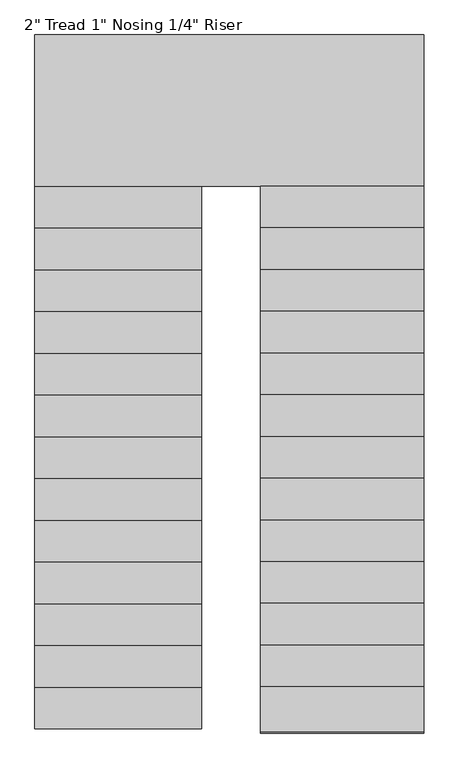
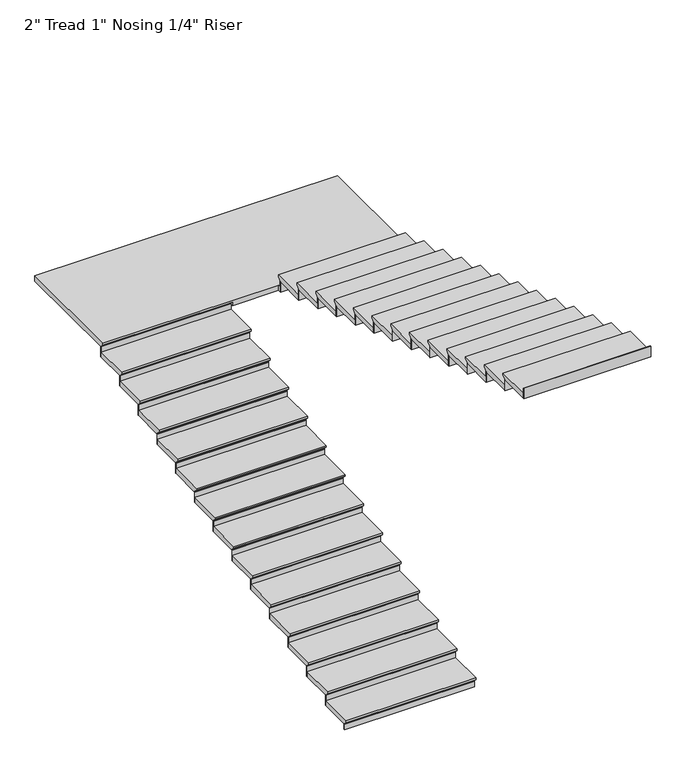
"""IFC4 building model written with IfcOpenShell, lengths in millimetres: stair flight geometry."""

from ifc_helpers import new_model, si_unit, origin, place, context, project, spatial, faceted_brep, source, transform, mapped, element, save


def stair_flight_f733c31e(model_context):
    return source(origin(), model_context, "Body", "Brep", [
        faceted_brep([(-629.5987998, 2564.5067329, 9685.5642857), (-629.5987998, 2564.5067329, 9704.6142857), (-1848.7987998, 2564.5067329, 9704.6142857), (-1848.7987998, 2564.5067329, 9685.5642857), (-629.5987998, 2589.9067329, 9660.1642857), (-1848.7987998, 2589.9067329, 9660.1642857), (-629.5987998, 2894.7067329, 9704.6142857), (-1848.7987998, 2894.7067329, 9704.6142857), (-1848.7987998, 2589.9067329, 9653.8142857), (-1848.7987998, 2894.7067329, 9653.8142857), (-629.5987998, 2894.7067329, 9653.8142857), (-629.5987998, 2589.9067329, 9653.8142857)], [[[0, 1, 2, 3]], [[4, 0, 3, 5]], [[2, 1, 6, 7]], [[8, 9, 10, 11]], [[2, 7, 9, 8, 5, 3]], [[8, 11, 4, 5]], [[6, 1, 0, 4, 11, 10]], [[7, 6, 10, 9]]]),
        faceted_brep([(-629.5987998, 2589.9067329, 9653.8142857), (-629.5987998, 2589.9067329, 9601.2), (-629.5987998, 2596.2567329, 9601.2), (-629.5987998, 2596.2567329, 9653.8142857), (-1848.7987998, 2589.9067329, 9653.8142857), (-1848.7987998, 2596.2567329, 9653.8142857), (-1848.7987998, 2596.2567329, 9601.2), (-1848.7987998, 2589.9067329, 9601.2)], [[[0, 1, 2, 3]], [[4, 5, 6, 7]], [[1, 0, 4, 7]], [[2, 1, 7, 6]], [[3, 2, 6, 5]], [[0, 3, 5, 4]]]),
        faceted_brep([(-629.5987998, 2894.7067329, 9757.2285714), (-629.5987998, 2894.7067329, 9653.8142857), (-629.5987998, 2901.0567329, 9653.8142857), (-629.5987998, 2901.0567329, 9757.2285714), (-1848.7987998, 2894.7067329, 9757.2285714), (-1848.7987998, 2901.0567329, 9757.2285714), (-1848.7987998, 2901.0567329, 9653.8142857), (-1848.7987998, 2894.7067329, 9653.8142857)], [[[0, 1, 2, 3]], [[4, 5, 6, 7]], [[1, 0, 4, 7]], [[2, 1, 7, 6]], [[3, 2, 6, 5]], [[0, 3, 5, 4]]]),
        faceted_brep([(-1848.7987998, 2869.3067329, 9808.0285714), (-629.5987998, 2869.3067329, 9808.0285714), (-629.5987998, 3199.5067329, 9808.0285714), (-1848.7987998, 3199.5067329, 9808.0285714), (-1848.7987998, 2894.7067329, 9757.2285714), (-1848.7987998, 3199.5067329, 9757.2285714), (-629.5987998, 3199.5067329, 9757.2285714), (-629.5987998, 2894.7067329, 9757.2285714), (-1848.7987998, 2894.7067329, 9763.5785714), (-1848.7987998, 2869.3067329, 9788.9785714), (-629.5987998, 2894.7067329, 9763.5785714), (-629.5987998, 2869.3067329, 9788.9785714)], [[[0, 1, 2, 3]], [[4, 5, 6, 7]], [[0, 3, 5, 4, 8, 9]], [[4, 7, 10, 8]], [[2, 1, 11, 10, 7, 6]], [[3, 2, 6, 5]], [[11, 1, 0, 9]], [[10, 11, 9, 8]]]),
        faceted_brep([(-629.5987998, 3199.5067329, 9860.6428571), (-629.5987998, 3199.5067329, 9757.2285714), (-629.5987998, 3205.8567329, 9757.2285714), (-629.5987998, 3205.8567329, 9860.6428571), (-1848.7987998, 3199.5067329, 9860.6428571), (-1848.7987998, 3205.8567329, 9860.6428571), (-1848.7987998, 3205.8567329, 9757.2285714), (-1848.7987998, 3199.5067329, 9757.2285714)], [[[0, 1, 2, 3]], [[4, 5, 6, 7]], [[1, 0, 4, 7]], [[2, 1, 7, 6]], [[3, 2, 6, 5]], [[0, 3, 5, 4]]]),
        faceted_brep([(-1848.7987998, 3174.1067329, 9911.4428571), (-629.5987998, 3174.1067329, 9911.4428571), (-629.5987998, 3504.3067329, 9911.4428571), (-1848.7987998, 3504.3067329, 9911.4428571), (-1848.7987998, 3199.5067329, 9860.6428571), (-1848.7987998, 3504.3067329, 9860.6428571), (-629.5987998, 3504.3067329, 9860.6428571), (-629.5987998, 3199.5067329, 9860.6428571), (-1848.7987998, 3199.5067329, 9866.9928571), (-1848.7987998, 3174.1067329, 9892.3928571), (-629.5987998, 3199.5067329, 9866.9928571), (-629.5987998, 3174.1067329, 9892.3928571)], [[[0, 1, 2, 3]], [[4, 5, 6, 7]], [[0, 3, 5, 4, 8, 9]], [[4, 7, 10, 8]], [[2, 1, 11, 10, 7, 6]], [[3, 2, 6, 5]], [[11, 1, 0, 9]], [[10, 11, 9, 8]]]),
        faceted_brep([(-629.5987998, 3504.3067329, 9964.0571429), (-629.5987998, 3504.3067329, 9860.6428571), (-629.5987998, 3510.6567329, 9860.6428571), (-629.5987998, 3510.6567329, 9964.0571429), (-1848.7987998, 3504.3067329, 9964.0571429), (-1848.7987998, 3510.6567329, 9964.0571429), (-1848.7987998, 3510.6567329, 9860.6428571), (-1848.7987998, 3504.3067329, 9860.6428571)], [[[0, 1, 2, 3]], [[4, 5, 6, 7]], [[1, 0, 4, 7]], [[2, 1, 7, 6]], [[3, 2, 6, 5]], [[0, 3, 5, 4]]]),
        faceted_brep([(-1848.7987998, 3478.9067329, 10014.8571429), (-629.5987998, 3478.9067329, 10014.8571429), (-629.5987998, 3809.1067329, 10014.8571429), (-1848.7987998, 3809.1067329, 10014.8571429), (-1848.7987998, 3504.3067329, 9964.0571429), (-1848.7987998, 3809.1067329, 9964.0571429), (-629.5987998, 3809.1067329, 9964.0571429), (-629.5987998, 3504.3067329, 9964.0571429), (-1848.7987998, 3504.3067329, 9970.4071429), (-1848.7987998, 3478.9067329, 9995.8071429), (-629.5987998, 3504.3067329, 9970.4071429), (-629.5987998, 3478.9067329, 9995.8071429)], [[[0, 1, 2, 3]], [[4, 5, 6, 7]], [[0, 3, 5, 4, 8, 9]], [[4, 7, 10, 8]], [[2, 1, 11, 10, 7, 6]], [[3, 2, 6, 5]], [[11, 1, 0, 9]], [[10, 11, 9, 8]]]),
        faceted_brep([(-629.5987998, 3809.1067329, 10067.4714286), (-629.5987998, 3809.1067329, 9964.0571429), (-629.5987998, 3815.4567329, 9964.0571429), (-629.5987998, 3815.4567329, 10067.4714286), (-1848.7987998, 3809.1067329, 10067.4714286), (-1848.7987998, 3815.4567329, 10067.4714286), (-1848.7987998, 3815.4567329, 9964.0571429), (-1848.7987998, 3809.1067329, 9964.0571429)], [[[0, 1, 2, 3]], [[4, 5, 6, 7]], [[1, 0, 4, 7]], [[2, 1, 7, 6]], [[3, 2, 6, 5]], [[0, 3, 5, 4]]]),
        faceted_brep([(-1848.7987998, 3783.7067329, 10118.2714286), (-629.5987998, 3783.7067329, 10118.2714286), (-629.5987998, 4113.9067329, 10118.2714286), (-1848.7987998, 4113.9067329, 10118.2714286), (-1848.7987998, 3809.1067329, 10067.4714286), (-1848.7987998, 4113.9067329, 10067.4714286), (-629.5987998, 4113.9067329, 10067.4714286), (-629.5987998, 3809.1067329, 10067.4714286), (-1848.7987998, 3809.1067329, 10073.8214286), (-1848.7987998, 3783.7067329, 10099.2214286), (-629.5987998, 3809.1067329, 10073.8214286), (-629.5987998, 3783.7067329, 10099.2214286)], [[[0, 1, 2, 3]], [[4, 5, 6, 7]], [[0, 3, 5, 4, 8, 9]], [[4, 7, 10, 8]], [[2, 1, 11, 10, 7, 6]], [[3, 2, 6, 5]], [[11, 1, 0, 9]], [[10, 11, 9, 8]]]),
        faceted_brep([(-629.5987998, 4113.9067329, 10170.8857143), (-629.5987998, 4113.9067329, 10067.4714286), (-629.5987998, 4120.2567329, 10067.4714286), (-629.5987998, 4120.2567329, 10170.8857143), (-1848.7987998, 4113.9067329, 10170.8857143), (-1848.7987998, 4120.2567329, 10170.8857143), (-1848.7987998, 4120.2567329, 10067.4714286), (-1848.7987998, 4113.9067329, 10067.4714286)], [[[0, 1, 2, 3]], [[4, 5, 6, 7]], [[1, 0, 4, 7]], [[2, 1, 7, 6]], [[3, 2, 6, 5]], [[0, 3, 5, 4]]]),
        faceted_brep([(-1848.7987998, 4088.5067329, 10221.6857143), (-629.5987998, 4088.5067329, 10221.6857143), (-629.5987998, 4418.7067329, 10221.6857143), (-1848.7987998, 4418.7067329, 10221.6857143), (-1848.7987998, 4113.9067329, 10170.8857143), (-1848.7987998, 4418.7067329, 10170.8857143), (-629.5987998, 4418.7067329, 10170.8857143), (-629.5987998, 4113.9067329, 10170.8857143), (-1848.7987998, 4113.9067329, 10177.2357143), (-1848.7987998, 4088.5067329, 10202.6357143), (-629.5987998, 4113.9067329, 10177.2357143), (-629.5987998, 4088.5067329, 10202.6357143)], [[[0, 1, 2, 3]], [[4, 5, 6, 7]], [[0, 3, 5, 4, 8, 9]], [[4, 7, 10, 8]], [[2, 1, 11, 10, 7, 6]], [[3, 2, 6, 5]], [[11, 1, 0, 9]], [[10, 11, 9, 8]]]),
        faceted_brep([(-629.5987998, 4418.7067329, 10274.3), (-629.5987998, 4418.7067329, 10170.8857143), (-629.5987998, 4425.0567329, 10170.8857143), (-629.5987998, 4425.0567329, 10274.3), (-1848.7987998, 4418.7067329, 10274.3), (-1848.7987998, 4425.0567329, 10274.3), (-1848.7987998, 4425.0567329, 10170.8857143), (-1848.7987998, 4418.7067329, 10170.8857143)], [[[0, 1, 2, 3]], [[4, 5, 6, 7]], [[1, 0, 4, 7]], [[2, 1, 7, 6]], [[3, 2, 6, 5]], [[0, 3, 5, 4]]]),
        faceted_brep([(-1848.7987998, 4393.3067329, 10325.1), (-629.5987998, 4393.3067329, 10325.1), (-629.5987998, 4723.5067329, 10325.1), (-1848.7987998, 4723.5067329, 10325.1), (-1848.7987998, 4418.7067329, 10274.3), (-1848.7987998, 4723.5067329, 10274.3), (-629.5987998, 4723.5067329, 10274.3), (-629.5987998, 4418.7067329, 10274.3), (-1848.7987998, 4418.7067329, 10280.65), (-1848.7987998, 4393.3067329, 10306.05), (-629.5987998, 4418.7067329, 10280.65), (-629.5987998, 4393.3067329, 10306.05)], [[[0, 1, 2, 3]], [[4, 5, 6, 7]], [[0, 3, 5, 4, 8, 9]], [[4, 7, 10, 8]], [[2, 1, 11, 10, 7, 6]], [[3, 2, 6, 5]], [[11, 1, 0, 9]], [[10, 11, 9, 8]]]),
        faceted_brep([(-629.5987998, 4723.5067329, 10377.7142857), (-629.5987998, 4723.5067329, 10274.3), (-629.5987998, 4729.8567329, 10274.3), (-629.5987998, 4729.8567329, 10377.7142857), (-1848.7987998, 4723.5067329, 10377.7142857), (-1848.7987998, 4729.8567329, 10377.7142857), (-1848.7987998, 4729.8567329, 10274.3), (-1848.7987998, 4723.5067329, 10274.3)], [[[0, 1, 2, 3]], [[4, 5, 6, 7]], [[1, 0, 4, 7]], [[2, 1, 7, 6]], [[3, 2, 6, 5]], [[0, 3, 5, 4]]]),
        faceted_brep([(-1848.7987998, 4698.1067329, 10428.5142857), (-629.5987998, 4698.1067329, 10428.5142857), (-629.5987998, 5028.3067329, 10428.5142857), (-1848.7987998, 5028.3067329, 10428.5142857), (-1848.7987998, 4723.5067329, 10377.7142857), (-1848.7987998, 5028.3067329, 10377.7142857), (-629.5987998, 5028.3067329, 10377.7142857), (-629.5987998, 4723.5067329, 10377.7142857), (-1848.7987998, 4723.5067329, 10384.0642857), (-1848.7987998, 4698.1067329, 10409.4642857), (-629.5987998, 4723.5067329, 10384.0642857), (-629.5987998, 4698.1067329, 10409.4642857)], [[[0, 1, 2, 3]], [[4, 5, 6, 7]], [[0, 3, 5, 4, 8, 9]], [[4, 7, 10, 8]], [[2, 1, 11, 10, 7, 6]], [[3, 2, 6, 5]], [[11, 1, 0, 9]], [[10, 11, 9, 8]]]),
        faceted_brep([(-629.5987998, 5028.3067329, 10481.1285714), (-629.5987998, 5028.3067329, 10377.7142857), (-629.5987998, 5034.6567329, 10377.7142857), (-629.5987998, 5034.6567329, 10481.1285714), (-1848.7987998, 5028.3067329, 10481.1285714), (-1848.7987998, 5034.6567329, 10481.1285714), (-1848.7987998, 5034.6567329, 10377.7142857), (-1848.7987998, 5028.3067329, 10377.7142857)], [[[0, 1, 2, 3]], [[4, 5, 6, 7]], [[1, 0, 4, 7]], [[2, 1, 7, 6]], [[3, 2, 6, 5]], [[0, 3, 5, 4]]]),
        faceted_brep([(-1848.7987998, 5002.9067329, 10531.9285714), (-629.5987998, 5002.9067329, 10531.9285714), (-629.5987998, 5333.1067329, 10531.9285714), (-1848.7987998, 5333.1067329, 10531.9285714), (-1848.7987998, 5028.3067329, 10481.1285714), (-1848.7987998, 5333.1067329, 10481.1285714), (-629.5987998, 5333.1067329, 10481.1285714), (-629.5987998, 5028.3067329, 10481.1285714), (-1848.7987998, 5028.3067329, 10487.4785714), (-1848.7987998, 5002.9067329, 10512.8785714), (-629.5987998, 5028.3067329, 10487.4785714), (-629.5987998, 5002.9067329, 10512.8785714)], [[[0, 1, 2, 3]], [[4, 5, 6, 7]], [[0, 3, 5, 4, 8, 9]], [[4, 7, 10, 8]], [[2, 1, 11, 10, 7, 6]], [[3, 2, 6, 5]], [[11, 1, 0, 9]], [[10, 11, 9, 8]]]),
        faceted_brep([(-629.5987998, 5333.1067329, 10584.5428571), (-629.5987998, 5333.1067329, 10481.1285714), (-629.5987998, 5339.4567329, 10481.1285714), (-629.5987998, 5339.4567329, 10584.5428571), (-1848.7987998, 5333.1067329, 10584.5428571), (-1848.7987998, 5339.4567329, 10584.5428571), (-1848.7987998, 5339.4567329, 10481.1285714), (-1848.7987998, 5333.1067329, 10481.1285714)], [[[0, 1, 2, 3]], [[4, 5, 6, 7]], [[1, 0, 4, 7]], [[2, 1, 7, 6]], [[3, 2, 6, 5]], [[0, 3, 5, 4]]]),
        faceted_brep([(-1848.7987998, 5307.7067329, 10635.3428571), (-629.5987998, 5307.7067329, 10635.3428571), (-629.5987998, 5637.9067329, 10635.3428571), (-1848.7987998, 5637.9067329, 10635.3428571), (-1848.7987998, 5333.1067329, 10584.5428571), (-1848.7987998, 5637.9067329, 10584.5428571), (-629.5987998, 5637.9067329, 10584.5428571), (-629.5987998, 5333.1067329, 10584.5428571), (-1848.7987998, 5333.1067329, 10590.8928571), (-1848.7987998, 5307.7067329, 10616.2928571), (-629.5987998, 5333.1067329, 10590.8928571), (-629.5987998, 5307.7067329, 10616.2928571)], [[[0, 1, 2, 3]], [[4, 5, 6, 7]], [[0, 3, 5, 4, 8, 9]], [[4, 7, 10, 8]], [[2, 1, 11, 10, 7, 6]], [[3, 2, 6, 5]], [[11, 1, 0, 9]], [[10, 11, 9, 8]]]),
        faceted_brep([(-629.5987998, 5637.9067329, 10687.9571429), (-629.5987998, 5637.9067329, 10584.5428571), (-629.5987998, 5644.2567329, 10584.5428571), (-629.5987998, 5644.2567329, 10687.9571429), (-1848.7987998, 5637.9067329, 10687.9571429), (-1848.7987998, 5644.2567329, 10687.9571429), (-1848.7987998, 5644.2567329, 10584.5428571), (-1848.7987998, 5637.9067329, 10584.5428571)], [[[0, 1, 2, 3]], [[4, 5, 6, 7]], [[1, 0, 4, 7]], [[2, 1, 7, 6]], [[3, 2, 6, 5]], [[0, 3, 5, 4]]]),
        faceted_brep([(-1848.7987998, 5612.5067329, 10738.7571429), (-629.5987998, 5612.5067329, 10738.7571429), (-629.5987998, 5942.7067329, 10738.7571429), (-1848.7987998, 5942.7067329, 10738.7571429), (-1848.7987998, 5637.9067329, 10687.9571429), (-1848.7987998, 5942.7067329, 10687.9571429), (-629.5987998, 5942.7067329, 10687.9571429), (-629.5987998, 5637.9067329, 10687.9571429), (-1848.7987998, 5637.9067329, 10694.3071429), (-1848.7987998, 5612.5067329, 10719.7071429), (-629.5987998, 5637.9067329, 10694.3071429), (-629.5987998, 5612.5067329, 10719.7071429)], [[[0, 1, 2, 3]], [[4, 5, 6, 7]], [[0, 3, 5, 4, 8, 9]], [[4, 7, 10, 8]], [[2, 1, 11, 10, 7, 6]], [[3, 2, 6, 5]], [[11, 1, 0, 9]], [[10, 11, 9, 8]]]),
        faceted_brep([(-629.5987998, 5942.7067329, 10791.3714286), (-629.5987998, 5942.7067329, 10687.9571429), (-629.5987998, 5949.0567329, 10687.9571429), (-629.5987998, 5949.0567329, 10791.3714286), (-1848.7987998, 5942.7067329, 10791.3714286), (-1848.7987998, 5949.0567329, 10791.3714286), (-1848.7987998, 5949.0567329, 10687.9571429), (-1848.7987998, 5942.7067329, 10687.9571429)], [[[0, 1, 2, 3]], [[4, 5, 6, 7]], [[1, 0, 4, 7]], [[2, 1, 7, 6]], [[3, 2, 6, 5]], [[0, 3, 5, 4]]]),
        faceted_brep([(-1848.7987998, 5917.3067329, 10842.1714286), (-629.5987998, 5917.3067329, 10842.1714286), (-629.5987998, 6247.5067329, 10842.1714286), (-1848.7987998, 6247.5067329, 10842.1714286), (-1848.7987998, 5942.7067329, 10791.3714286), (-1848.7987998, 6247.5067329, 10791.3714286), (-629.5987998, 6247.5067329, 10791.3714286), (-629.5987998, 5942.7067329, 10791.3714286), (-1848.7987998, 5942.7067329, 10797.7214286), (-1848.7987998, 5917.3067329, 10823.1214286), (-629.5987998, 5942.7067329, 10797.7214286), (-629.5987998, 5917.3067329, 10823.1214286)], [[[0, 1, 2, 3]], [[4, 5, 6, 7]], [[0, 3, 5, 4, 8, 9]], [[4, 7, 10, 8]], [[2, 1, 11, 10, 7, 6]], [[3, 2, 6, 5]], [[11, 1, 0, 9]], [[10, 11, 9, 8]]]),
        faceted_brep([(-629.5987998, 6247.5067329, 10894.7857143), (-629.5987998, 6247.5067329, 10791.3714286), (-629.5987998, 6253.8567329, 10791.3714286), (-629.5987998, 6253.8567329, 10894.7857143), (-1848.7987998, 6247.5067329, 10894.7857143), (-1848.7987998, 6253.8567329, 10894.7857143), (-1848.7987998, 6253.8567329, 10791.3714286), (-1848.7987998, 6247.5067329, 10791.3714286)], [[[0, 1, 2, 3]], [[4, 5, 6, 7]], [[1, 0, 4, 7]], [[2, 1, 7, 6]], [[3, 2, 6, 5]], [[0, 3, 5, 4]]]),
        faceted_brep([(-1848.7987998, 6222.1067329, 10945.5857143), (-629.5987998, 6222.1067329, 10945.5857143), (-629.5987998, 6552.3067329, 10945.5857143), (-1848.7987998, 6552.3067329, 10945.5857143), (-1848.7987998, 6247.5067329, 10894.7857143), (-1848.7987998, 6552.3067329, 10894.7857143), (-629.5987998, 6552.3067329, 10894.7857143), (-629.5987998, 6247.5067329, 10894.7857143), (-1848.7987998, 6247.5067329, 10901.1357143), (-1848.7987998, 6222.1067329, 10926.5357143), (-629.5987998, 6247.5067329, 10901.1357143), (-629.5987998, 6222.1067329, 10926.5357143)], [[[0, 1, 2, 3]], [[4, 5, 6, 7]], [[0, 3, 5, 4, 8, 9]], [[4, 7, 10, 8]], [[2, 1, 11, 10, 7, 6]], [[3, 2, 6, 5]], [[11, 1, 0, 9]], [[10, 11, 9, 8]]]),
        faceted_brep([(-629.5987998, 6552.3067329, 10998.2), (-629.5987998, 6552.3067329, 10894.7857143), (-629.5987998, 6558.6567329, 10894.7857143), (-629.5987998, 6558.6567329, 10998.2), (-1848.7987998, 6552.3067329, 10998.2), (-1848.7987998, 6558.6567329, 10998.2), (-1848.7987998, 6558.6567329, 10894.7857143), (-1848.7987998, 6552.3067329, 10894.7857143)], [[[0, 1, 2, 3]], [[4, 5, 6, 7]], [[1, 0, 4, 7]], [[2, 1, 7, 6]], [[3, 2, 6, 5]], [[0, 3, 5, 4]]]),
        faceted_brep([(996.0012002, 6501.5067329, 11049.0), (996.0012002, 7631.8067329, 11049.0), (-1848.7987998, 7631.8067329, 11049.0), (-1848.7987998, 6526.9067329, 11049.0), (-197.7987915, 6526.9067329, 11049.0), (-197.7987915, 6501.5067329, 11049.0), (996.0012002, 7631.8067329, 10998.2), (996.0012002, 6501.5067329, 10998.2), (-197.7987915, 6501.5067329, 10998.2), (-197.7987915, 6526.9067329, 10998.2), (-629.5987998, 6526.9067329, 10998.2), (-629.5987998, 6552.3067329, 10998.2), (-1848.7987998, 6552.3067329, 10998.2), (-1848.7987998, 7631.8067329, 10998.2), (-629.5987998, 6552.3067329, 11004.55), (-1848.7987998, 6552.3067329, 11004.55), (-1848.7987998, 6526.9067329, 11029.95), (-629.5987998, 6526.9067329, 11029.95)], [[[0, 1, 2, 3, 4, 5]], [[6, 7, 8, 9, 10, 11, 12, 13]], [[1, 0, 7, 6]], [[2, 1, 6, 13]], [[12, 11, 14, 15]], [[4, 3, 16, 17, 10, 9]], [[5, 4, 9, 8]], [[0, 5, 8, 7]], [[16, 15, 14, 17]], [[3, 2, 13, 12, 15, 16]], [[11, 10, 17, 14]]]),
        faceted_brep([(-197.7987915, 6501.5067329, 11101.6142857), (-197.7987915, 6501.5067329, 10998.2), (-197.7987915, 6495.1567329, 10998.2), (-197.7987915, 6495.1567329, 11101.6142857), (996.0012002, 6501.5067329, 11101.6142857), (996.0012002, 6495.1567329, 11101.6142857), (996.0012002, 6495.1567329, 10998.2), (996.0012002, 6501.5067329, 10998.2)], [[[0, 1, 2, 3]], [[4, 5, 6, 7]], [[1, 0, 4, 7]], [[2, 1, 7, 6]], [[3, 2, 6, 5]], [[0, 3, 5, 4]]]),
        faceted_brep([(996.0012002, 6526.9067329, 11152.4142857), (-197.7987915, 6526.9067329, 11152.4142857), (-197.7987915, 6196.7067329, 11152.4142857), (996.0012002, 6196.7067329, 11152.4142857), (996.0012002, 6501.5067329, 11101.6142857), (996.0012002, 6196.7067329, 11101.6142857), (-197.7987915, 6196.7067329, 11101.6142857), (-197.7987915, 6501.5067329, 11101.6142857), (996.0012002, 6501.5067329, 11107.9642857), (996.0012002, 6526.9067329, 11133.3642857), (-197.7987915, 6501.5067329, 11107.9642857), (-197.7987915, 6526.9067329, 11133.3642857)], [[[0, 1, 2, 3]], [[4, 5, 6, 7]], [[0, 3, 5, 4, 8, 9]], [[4, 7, 10, 8]], [[2, 1, 11, 10, 7, 6]], [[3, 2, 6, 5]], [[11, 1, 0, 9]], [[10, 11, 9, 8]]]),
        faceted_brep([(-197.7987915, 6196.7067329, 11205.0285714), (-197.7987915, 6196.7067329, 11101.6142857), (-197.7987915, 6190.3567329, 11101.6142857), (-197.7987915, 6190.3567329, 11205.0285714), (996.0012002, 6196.7067329, 11205.0285714), (996.0012002, 6190.3567329, 11205.0285714), (996.0012002, 6190.3567329, 11101.6142857), (996.0012002, 6196.7067329, 11101.6142857)], [[[0, 1, 2, 3]], [[4, 5, 6, 7]], [[1, 0, 4, 7]], [[2, 1, 7, 6]], [[3, 2, 6, 5]], [[0, 3, 5, 4]]]),
        faceted_brep([(996.0012002, 6222.1067329, 11255.8285714), (-197.7987915, 6222.1067329, 11255.8285714), (-197.7987915, 5891.9067329, 11255.8285714), (996.0012002, 5891.9067329, 11255.8285714), (996.0012002, 6196.7067329, 11205.0285714), (996.0012002, 5891.9067329, 11205.0285714), (-197.7987915, 5891.9067329, 11205.0285714), (-197.7987915, 6196.7067329, 11205.0285714), (996.0012002, 6196.7067329, 11211.3785714), (996.0012002, 6222.1067329, 11236.7785714), (-197.7987915, 6196.7067329, 11211.3785714), (-197.7987915, 6222.1067329, 11236.7785714)], [[[0, 1, 2, 3]], [[4, 5, 6, 7]], [[0, 3, 5, 4, 8, 9]], [[4, 7, 10, 8]], [[2, 1, 11, 10, 7, 6]], [[3, 2, 6, 5]], [[11, 1, 0, 9]], [[10, 11, 9, 8]]]),
        faceted_brep([(-197.7987915, 5891.9067329, 11308.4428571), (-197.7987915, 5891.9067329, 11205.0285714), (-197.7987915, 5885.5567329, 11205.0285714), (-197.7987915, 5885.5567329, 11308.4428571), (996.0012002, 5891.9067329, 11308.4428571), (996.0012002, 5885.5567329, 11308.4428571), (996.0012002, 5885.5567329, 11205.0285714), (996.0012002, 5891.9067329, 11205.0285714)], [[[0, 1, 2, 3]], [[4, 5, 6, 7]], [[1, 0, 4, 7]], [[2, 1, 7, 6]], [[3, 2, 6, 5]], [[0, 3, 5, 4]]]),
        faceted_brep([(996.0012002, 5917.3067329, 11359.2428571), (-197.7987915, 5917.3067329, 11359.2428571), (-197.7987915, 5587.1067329, 11359.2428571), (996.0012002, 5587.1067329, 11359.2428571), (996.0012002, 5891.9067329, 11308.4428571), (996.0012002, 5587.1067329, 11308.4428571), (-197.7987915, 5587.1067329, 11308.4428571), (-197.7987915, 5891.9067329, 11308.4428571), (996.0012002, 5891.9067329, 11314.7928571), (996.0012002, 5917.3067329, 11340.1928571), (-197.7987915, 5891.9067329, 11314.7928571), (-197.7987915, 5917.3067329, 11340.1928571)], [[[0, 1, 2, 3]], [[4, 5, 6, 7]], [[0, 3, 5, 4, 8, 9]], [[4, 7, 10, 8]], [[2, 1, 11, 10, 7, 6]], [[3, 2, 6, 5]], [[11, 1, 0, 9]], [[10, 11, 9, 8]]]),
        faceted_brep([(-197.7987915, 5587.1067329, 11411.8571429), (-197.7987915, 5587.1067329, 11308.4428571), (-197.7987915, 5580.7567329, 11308.4428571), (-197.7987915, 5580.7567329, 11411.8571429), (996.0012002, 5587.1067329, 11411.8571429), (996.0012002, 5580.7567329, 11411.8571429), (996.0012002, 5580.7567329, 11308.4428571), (996.0012002, 5587.1067329, 11308.4428571)], [[[0, 1, 2, 3]], [[4, 5, 6, 7]], [[1, 0, 4, 7]], [[2, 1, 7, 6]], [[3, 2, 6, 5]], [[0, 3, 5, 4]]]),
        faceted_brep([(996.0012002, 5612.5067329, 11462.6571429), (-197.7987915, 5612.5067329, 11462.6571429), (-197.7987915, 5282.3067329, 11462.6571429), (996.0012002, 5282.3067329, 11462.6571429), (996.0012002, 5587.1067329, 11411.8571429), (996.0012002, 5282.3067329, 11411.8571429), (-197.7987915, 5282.3067329, 11411.8571429), (-197.7987915, 5587.1067329, 11411.8571429), (996.0012002, 5587.1067329, 11418.2071429), (996.0012002, 5612.5067329, 11443.6071429), (-197.7987915, 5587.1067329, 11418.2071429), (-197.7987915, 5612.5067329, 11443.6071429)], [[[0, 1, 2, 3]], [[4, 5, 6, 7]], [[0, 3, 5, 4, 8, 9]], [[4, 7, 10, 8]], [[2, 1, 11, 10, 7, 6]], [[3, 2, 6, 5]], [[11, 1, 0, 9]], [[10, 11, 9, 8]]]),
        faceted_brep([(-197.7987915, 5282.3067329, 11515.2714286), (-197.7987915, 5282.3067329, 11411.8571429), (-197.7987915, 5275.9567329, 11411.8571429), (-197.7987915, 5275.9567329, 11515.2714286), (996.0012002, 5282.3067329, 11515.2714286), (996.0012002, 5275.9567329, 11515.2714286), (996.0012002, 5275.9567329, 11411.8571429), (996.0012002, 5282.3067329, 11411.8571429)], [[[0, 1, 2, 3]], [[4, 5, 6, 7]], [[1, 0, 4, 7]], [[2, 1, 7, 6]], [[3, 2, 6, 5]], [[0, 3, 5, 4]]]),
        faceted_brep([(996.0012002, 5307.7067329, 11566.0714286), (-197.7987915, 5307.7067329, 11566.0714286), (-197.7987915, 4977.5067329, 11566.0714286), (996.0012002, 4977.5067329, 11566.0714286), (996.0012002, 5282.3067329, 11515.2714286), (996.0012002, 4977.5067329, 11515.2714286), (-197.7987915, 4977.5067329, 11515.2714286), (-197.7987915, 5282.3067329, 11515.2714286), (996.0012002, 5282.3067329, 11521.6214286), (996.0012002, 5307.7067329, 11547.0214286), (-197.7987915, 5282.3067329, 11521.6214286), (-197.7987915, 5307.7067329, 11547.0214286)], [[[0, 1, 2, 3]], [[4, 5, 6, 7]], [[0, 3, 5, 4, 8, 9]], [[4, 7, 10, 8]], [[2, 1, 11, 10, 7, 6]], [[3, 2, 6, 5]], [[11, 1, 0, 9]], [[10, 11, 9, 8]]]),
        faceted_brep([(-197.7987915, 4977.5067329, 11618.6857143), (-197.7987915, 4977.5067329, 11515.2714286), (-197.7987915, 4971.1567329, 11515.2714286), (-197.7987915, 4971.1567329, 11618.6857143), (996.0012002, 4977.5067329, 11618.6857143), (996.0012002, 4971.1567329, 11618.6857143), (996.0012002, 4971.1567329, 11515.2714286), (996.0012002, 4977.5067329, 11515.2714286)], [[[0, 1, 2, 3]], [[4, 5, 6, 7]], [[1, 0, 4, 7]], [[2, 1, 7, 6]], [[3, 2, 6, 5]], [[0, 3, 5, 4]]]),
        faceted_brep([(996.0012002, 5002.9067329, 11669.4857143), (-197.7987915, 5002.9067329, 11669.4857143), (-197.7987915, 4672.7067329, 11669.4857143), (996.0012002, 4672.7067329, 11669.4857143), (996.0012002, 4977.5067329, 11618.6857143), (996.0012002, 4672.7067329, 11618.6857143), (-197.7987915, 4672.7067329, 11618.6857143), (-197.7987915, 4977.5067329, 11618.6857143), (996.0012002, 4977.5067329, 11625.0357143), (996.0012002, 5002.9067329, 11650.4357143), (-197.7987915, 4977.5067329, 11625.0357143), (-197.7987915, 5002.9067329, 11650.4357143)], [[[0, 1, 2, 3]], [[4, 5, 6, 7]], [[0, 3, 5, 4, 8, 9]], [[4, 7, 10, 8]], [[2, 1, 11, 10, 7, 6]], [[3, 2, 6, 5]], [[11, 1, 0, 9]], [[10, 11, 9, 8]]]),
        faceted_brep([(-197.7987915, 4672.7067329, 11722.1), (-197.7987915, 4672.7067329, 11618.6857143), (-197.7987915, 4666.3567329, 11618.6857143), (-197.7987915, 4666.3567329, 11722.1), (996.0012002, 4672.7067329, 11722.1), (996.0012002, 4666.3567329, 11722.1), (996.0012002, 4666.3567329, 11618.6857143), (996.0012002, 4672.7067329, 11618.6857143)], [[[0, 1, 2, 3]], [[4, 5, 6, 7]], [[1, 0, 4, 7]], [[2, 1, 7, 6]], [[3, 2, 6, 5]], [[0, 3, 5, 4]]]),
        faceted_brep([(996.0012002, 4698.1067329, 11772.9), (-197.7987915, 4698.1067329, 11772.9), (-197.7987915, 4367.9067329, 11772.9), (996.0012002, 4367.9067329, 11772.9), (996.0012002, 4672.7067329, 11722.1), (996.0012002, 4367.9067329, 11722.1), (-197.7987915, 4367.9067329, 11722.1), (-197.7987915, 4672.7067329, 11722.1), (996.0012002, 4672.7067329, 11728.45), (996.0012002, 4698.1067329, 11753.85), (-197.7987915, 4672.7067329, 11728.45), (-197.7987915, 4698.1067329, 11753.85)], [[[0, 1, 2, 3]], [[4, 5, 6, 7]], [[0, 3, 5, 4, 8, 9]], [[4, 7, 10, 8]], [[2, 1, 11, 10, 7, 6]], [[3, 2, 6, 5]], [[11, 1, 0, 9]], [[10, 11, 9, 8]]]),
        faceted_brep([(-197.7987915, 4367.9067329, 11825.5142857), (-197.7987915, 4367.9067329, 11722.1), (-197.7987915, 4361.5567329, 11722.1), (-197.7987915, 4361.5567329, 11825.5142857), (996.0012002, 4367.9067329, 11825.5142857), (996.0012002, 4361.5567329, 11825.5142857), (996.0012002, 4361.5567329, 11722.1), (996.0012002, 4367.9067329, 11722.1)], [[[0, 1, 2, 3]], [[4, 5, 6, 7]], [[1, 0, 4, 7]], [[2, 1, 7, 6]], [[3, 2, 6, 5]], [[0, 3, 5, 4]]]),
        faceted_brep([(996.0012002, 4393.3067329, 11876.3142857), (-197.7987915, 4393.3067329, 11876.3142857), (-197.7987915, 4063.1067329, 11876.3142857), (996.0012002, 4063.1067329, 11876.3142857), (996.0012002, 4367.9067329, 11825.5142857), (996.0012002, 4063.1067329, 11825.5142857), (-197.7987915, 4063.1067329, 11825.5142857), (-197.7987915, 4367.9067329, 11825.5142857), (996.0012002, 4367.9067329, 11831.8642857), (996.0012002, 4393.3067329, 11857.2642857), (-197.7987915, 4367.9067329, 11831.8642857), (-197.7987915, 4393.3067329, 11857.2642857)], [[[0, 1, 2, 3]], [[4, 5, 6, 7]], [[0, 3, 5, 4, 8, 9]], [[4, 7, 10, 8]], [[2, 1, 11, 10, 7, 6]], [[3, 2, 6, 5]], [[11, 1, 0, 9]], [[10, 11, 9, 8]]]),
        faceted_brep([(-197.7987915, 4063.1067329, 11928.9285714), (-197.7987915, 4063.1067329, 11825.5142857), (-197.7987915, 4056.7567329, 11825.5142857), (-197.7987915, 4056.7567329, 11928.9285714), (996.0012002, 4063.1067329, 11928.9285714), (996.0012002, 4056.7567329, 11928.9285714), (996.0012002, 4056.7567329, 11825.5142857), (996.0012002, 4063.1067329, 11825.5142857)], [[[0, 1, 2, 3]], [[4, 5, 6, 7]], [[1, 0, 4, 7]], [[2, 1, 7, 6]], [[3, 2, 6, 5]], [[0, 3, 5, 4]]]),
        faceted_brep([(996.0012002, 4088.5067329, 11979.7285714), (-197.7987915, 4088.5067329, 11979.7285714), (-197.7987915, 3758.3067329, 11979.7285714), (996.0012002, 3758.3067329, 11979.7285714), (996.0012002, 4063.1067329, 11928.9285714), (996.0012002, 3758.3067329, 11928.9285714), (-197.7987915, 3758.3067329, 11928.9285714), (-197.7987915, 4063.1067329, 11928.9285714), (996.0012002, 4063.1067329, 11935.2785714), (996.0012002, 4088.5067329, 11960.6785714), (-197.7987915, 4063.1067329, 11935.2785714), (-197.7987915, 4088.5067329, 11960.6785714)], [[[0, 1, 2, 3]], [[4, 5, 6, 7]], [[0, 3, 5, 4, 8, 9]], [[4, 7, 10, 8]], [[2, 1, 11, 10, 7, 6]], [[3, 2, 6, 5]], [[11, 1, 0, 9]], [[10, 11, 9, 8]]]),
        faceted_brep([(-197.7987915, 3758.3067329, 12032.3428571), (-197.7987915, 3758.3067329, 11928.9285714), (-197.7987915, 3751.9567329, 11928.9285714), (-197.7987915, 3751.9567329, 12032.3428571), (996.0012002, 3758.3067329, 12032.3428571), (996.0012002, 3751.9567329, 12032.3428571), (996.0012002, 3751.9567329, 11928.9285714), (996.0012002, 3758.3067329, 11928.9285714)], [[[0, 1, 2, 3]], [[4, 5, 6, 7]], [[1, 0, 4, 7]], [[2, 1, 7, 6]], [[3, 2, 6, 5]], [[0, 3, 5, 4]]]),
        faceted_brep([(996.0012002, 3783.7067329, 12083.1428571), (-197.7987915, 3783.7067329, 12083.1428571), (-197.7987915, 3453.5067329, 12083.1428571), (996.0012002, 3453.5067329, 12083.1428571), (996.0012002, 3758.3067329, 12032.3428571), (996.0012002, 3453.5067329, 12032.3428571), (-197.7987915, 3453.5067329, 12032.3428571), (-197.7987915, 3758.3067329, 12032.3428571), (996.0012002, 3758.3067329, 12038.6928571), (996.0012002, 3783.7067329, 12064.0928571), (-197.7987915, 3758.3067329, 12038.6928571), (-197.7987915, 3783.7067329, 12064.0928571)], [[[0, 1, 2, 3]], [[4, 5, 6, 7]], [[0, 3, 5, 4, 8, 9]], [[4, 7, 10, 8]], [[2, 1, 11, 10, 7, 6]], [[3, 2, 6, 5]], [[11, 1, 0, 9]], [[10, 11, 9, 8]]]),
        faceted_brep([(-197.7987915, 3453.5067329, 12135.7571429), (-197.7987915, 3453.5067329, 12032.3428571), (-197.7987915, 3447.1567329, 12032.3428571), (-197.7987915, 3447.1567329, 12135.7571429), (996.0012002, 3453.5067329, 12135.7571429), (996.0012002, 3447.1567329, 12135.7571429), (996.0012002, 3447.1567329, 12032.3428571), (996.0012002, 3453.5067329, 12032.3428571)], [[[0, 1, 2, 3]], [[4, 5, 6, 7]], [[1, 0, 4, 7]], [[2, 1, 7, 6]], [[3, 2, 6, 5]], [[0, 3, 5, 4]]]),
        faceted_brep([(996.0012002, 3478.9067329, 12186.5571429), (-197.7987915, 3478.9067329, 12186.5571429), (-197.7987915, 3148.7067329, 12186.5571429), (996.0012002, 3148.7067329, 12186.5571429), (996.0012002, 3453.5067329, 12135.7571429), (996.0012002, 3148.7067329, 12135.7571429), (-197.7987915, 3148.7067329, 12135.7571429), (-197.7987915, 3453.5067329, 12135.7571429), (996.0012002, 3453.5067329, 12142.1071429), (996.0012002, 3478.9067329, 12167.5071429), (-197.7987915, 3453.5067329, 12142.1071429), (-197.7987915, 3478.9067329, 12167.5071429)], [[[0, 1, 2, 3]], [[4, 5, 6, 7]], [[0, 3, 5, 4, 8, 9]], [[4, 7, 10, 8]], [[2, 1, 11, 10, 7, 6]], [[3, 2, 6, 5]], [[11, 1, 0, 9]], [[10, 11, 9, 8]]]),
        faceted_brep([(-197.7987915, 3148.7067329, 12239.1714286), (-197.7987915, 3148.7067329, 12135.7571429), (-197.7987915, 3142.3567329, 12135.7571429), (-197.7987915, 3142.3567329, 12239.1714286), (996.0012002, 3148.7067329, 12239.1714286), (996.0012002, 3142.3567329, 12239.1714286), (996.0012002, 3142.3567329, 12135.7571429), (996.0012002, 3148.7067329, 12135.7571429)], [[[0, 1, 2, 3]], [[4, 5, 6, 7]], [[1, 0, 4, 7]], [[2, 1, 7, 6]], [[3, 2, 6, 5]], [[0, 3, 5, 4]]]),
        faceted_brep([(996.0012002, 3174.1067329, 12289.9714286), (-197.7987915, 3174.1067329, 12289.9714286), (-197.7987915, 2843.9067329, 12289.9714286), (996.0012002, 2843.9067329, 12289.9714286), (996.0012002, 3148.7067329, 12239.1714286), (996.0012002, 2843.9067329, 12239.1714286), (-197.7987915, 2843.9067329, 12239.1714286), (-197.7987915, 3148.7067329, 12239.1714286), (996.0012002, 3148.7067329, 12245.5214286), (996.0012002, 3174.1067329, 12270.9214286), (-197.7987915, 3148.7067329, 12245.5214286), (-197.7987915, 3174.1067329, 12270.9214286)], [[[0, 1, 2, 3]], [[4, 5, 6, 7]], [[0, 3, 5, 4, 8, 9]], [[4, 7, 10, 8]], [[2, 1, 11, 10, 7, 6]], [[3, 2, 6, 5]], [[11, 1, 0, 9]], [[10, 11, 9, 8]]]),
        faceted_brep([(-197.7987915, 2843.9067329, 12342.5857143), (-197.7987915, 2843.9067329, 12239.1714286), (-197.7987915, 2837.5567329, 12239.1714286), (-197.7987915, 2837.5567329, 12342.5857143), (996.0012002, 2843.9067329, 12342.5857143), (996.0012002, 2837.5567329, 12342.5857143), (996.0012002, 2837.5567329, 12239.1714286), (996.0012002, 2843.9067329, 12239.1714286)], [[[0, 1, 2, 3]], [[4, 5, 6, 7]], [[1, 0, 4, 7]], [[2, 1, 7, 6]], [[3, 2, 6, 5]], [[0, 3, 5, 4]]]),
        faceted_brep([(-197.7987915, 2539.1067329, 12446.0), (-197.7987915, 2539.1067329, 12342.5857143), (-197.7987915, 2532.7567329, 12342.5857143), (-197.7987915, 2532.7567329, 12446.0), (996.0012002, 2539.1067329, 12446.0), (996.0012002, 2532.7567329, 12446.0), (996.0012002, 2532.7567329, 12342.5857143), (996.0012002, 2539.1067329, 12342.5857143)], [[[0, 1, 2, 3]], [[4, 5, 6, 7]], [[1, 0, 4, 7]], [[2, 1, 7, 6]], [[3, 2, 6, 5]], [[0, 3, 5, 4]]]),
        faceted_brep([(996.0012002, 2869.3067329, 12393.3857143), (-197.7987915, 2869.3067329, 12393.3857143), (-197.7987915, 2539.1067329, 12393.3857143), (996.0012002, 2539.1067329, 12393.3857143), (996.0012002, 2843.9067329, 12342.5857143), (996.0012002, 2539.1067329, 12342.5857143), (-197.7987915, 2539.1067329, 12342.5857143), (-197.7987915, 2843.9067329, 12342.5857143), (996.0012002, 2843.9067329, 12348.9357143), (996.0012002, 2869.3067329, 12374.3357143), (-197.7987915, 2843.9067329, 12348.9357143), (-197.7987915, 2869.3067329, 12374.3357143)], [[[0, 1, 2, 3]], [[4, 5, 6, 7]], [[0, 3, 5, 4, 8, 9]], [[4, 7, 10, 8]], [[2, 1, 11, 10, 7, 6]], [[3, 2, 6, 5]], [[11, 1, 0, 9]], [[10, 11, 9, 8]]]),
    ])


if __name__ == "__main__":
    model = new_model("IFC4")
    model_context = context("Model", 3, world=origin())
    ifc_project = project(units=[si_unit("LENGTHUNIT", "METRE", prefix="MILLI")], contexts=[model_context])
    site = spatial("IfcSite", under=ifc_project)
    building = spatial("IfcBuilding", under=site)
    placement = place(None, origin())
    stair_flight_shape = stair_flight_f733c31e(model_context)
    element("IfcStairFlight", 1, ObjectType="2\" Tread 1\" Nosing 1/4\" Riser", at=placement, inside=building, context=model_context, shape_type="MappedRepresentation", body=[
        mapped(stair_flight_shape, transform((0.0, 0.0, 0.0), x_axis=(1.0, 0.0, 0.0), y_axis=(0.0, 1.0, 0.0), z_axis=(0.0, 0.0, 1.0))),
    ])
    save(model, "model.ifc")
